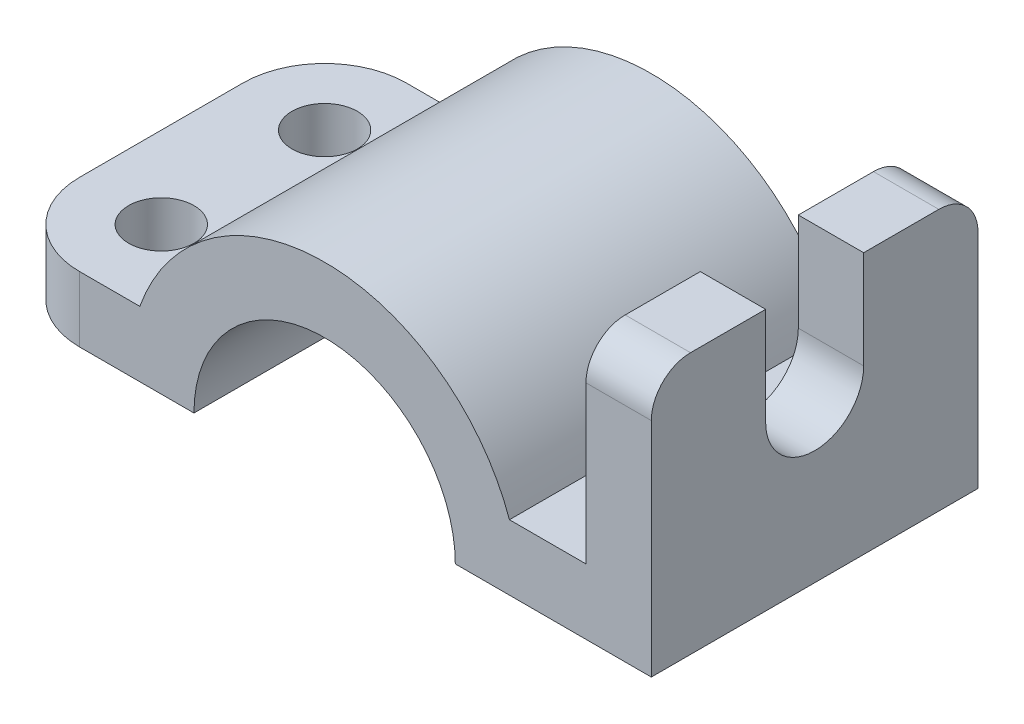
ISO-10303-21;
HEADER;
FILE_DESCRIPTION(('STEP AP214'),'2;1');
FILE_NAME('part.step','',(''),(''),'','','');
FILE_SCHEMA(('AUTOMOTIVE_DESIGN { 1 0 10303 214 1 1 1 1 }'));
ENDSEC;
DATA;
#1=APPLICATION_CONTEXT('core data for automotive mechanical design processes');
#2=APPLICATION_PROTOCOL_DEFINITION('international standard','automotive_design',2000,#1);
#3=PRODUCT_CONTEXT('',#1,'mechanical');
#4=PRODUCT('Part','Part','',(#3));
#5=PRODUCT_RELATED_PRODUCT_CATEGORY('part','',(#4));
#6=PRODUCT_DEFINITION_FORMATION('','',#4);
#7=PRODUCT_DEFINITION_CONTEXT('part definition',#1,'design');
#8=PRODUCT_DEFINITION('design','',#6,#7);
#9=PRODUCT_DEFINITION_SHAPE('','',#8);
#10=(LENGTH_UNIT() NAMED_UNIT(*) SI_UNIT(.MILLI.,.METRE.));
#11=(NAMED_UNIT(*) PLANE_ANGLE_UNIT() SI_UNIT($,.RADIAN.));
#12=(NAMED_UNIT(*) SI_UNIT($,.STERADIAN.) SOLID_ANGLE_UNIT());
#13=UNCERTAINTY_MEASURE_WITH_UNIT(LENGTH_MEASURE(1.E-05),#10,'distance_accuracy_value','');
#14=(GEOMETRIC_REPRESENTATION_CONTEXT(3) GLOBAL_UNCERTAINTY_ASSIGNED_CONTEXT((#13)) GLOBAL_UNIT_ASSIGNED_CONTEXT((#10,
#11,#12)) REPRESENTATION_CONTEXT('',''));
#15=CARTESIAN_POINT('',(0.,0.,0.));
#16=DIRECTION('',(0.,0.,1.));
#17=DIRECTION('',(1.,0.,0.));
#18=AXIS2_PLACEMENT_3D('',#15,#16,#17);
#19=CARTESIAN_POINT('',(50.,40.,25.));
#20=DIRECTION('',(-1.,0.,0.));
#21=DIRECTION('',(0.,-1.,0.));
#22=AXIS2_PLACEMENT_3D('',#19,#20,#21);
#23=PLANE('',#22);
#24=DIRECTION('',(0.,-1.,0.));
#25=VECTOR('',#24,1.);
#26=CARTESIAN_POINT('',(50.,40.,7.5));
#27=LINE('',#26,#25);
#28=CARTESIAN_POINT('',(50.,40.,7.5));
#29=VERTEX_POINT('',#28);
#30=CARTESIAN_POINT('',(50.000006,25.,7.5));
#31=VERTEX_POINT('',#30);
#32=EDGE_CURVE('E374',#29,#31,#27,.T.);
#33=ORIENTED_EDGE('',*,*,#32,.F.);
#34=DIRECTION('',(0.,0.,-1.));
#35=VECTOR('',#34,1.);
#36=CARTESIAN_POINT('',(50.,40.,25.));
#37=LINE('',#36,#35);
#38=CARTESIAN_POINT('',(50.,40.,19.));
#39=VERTEX_POINT('',#38);
#40=EDGE_CURVE('E272',#39,#29,#37,.T.);
#41=ORIENTED_EDGE('',*,*,#40,.F.);
#42=CARTESIAN_POINT('',(50.,34.,19.));
#43=DIRECTION('',(-1.,0.,0.));
#44=DIRECTION('',(0.,-1.,0.));
#45=AXIS2_PLACEMENT_3D('',#42,#43,#44);
#46=CIRCLE('',#45,6.);
#47=CARTESIAN_POINT('',(50.,34.,25.));
#48=VERTEX_POINT('',#47);
#49=EDGE_CURVE('E178',#39,#48,#46,.F.);
#50=ORIENTED_EDGE('',*,*,#49,.T.);
#51=DIRECTION('',(0.,1.,0.));
#52=VECTOR('',#51,1.);
#53=CARTESIAN_POINT('',(50.,40.,25.));
#54=LINE('',#53,#52);
#55=CARTESIAN_POINT('',(50.,0.,25.));
#56=VERTEX_POINT('',#55);
#57=EDGE_CURVE('E271',#56,#48,#54,.T.);
#58=ORIENTED_EDGE('',*,*,#57,.F.);
#59=DIRECTION('',(0.,0.,-1.));
#60=VECTOR('',#59,1.);
#61=CARTESIAN_POINT('',(50.,0.,25.));
#62=LINE('',#61,#60);
#63=CARTESIAN_POINT('',(50.,0.,-25.));
#64=VERTEX_POINT('',#63);
#65=EDGE_CURVE('E190',#56,#64,#62,.T.);
#66=ORIENTED_EDGE('',*,*,#65,.T.);
#67=DIRECTION('',(0.,1.,0.));
#68=VECTOR('',#67,1.);
#69=CARTESIAN_POINT('',(50.,40.,-25.));
#70=LINE('',#69,#68);
#71=CARTESIAN_POINT('',(50.,34.,-25.));
#72=VERTEX_POINT('',#71);
#73=EDGE_CURVE('E168',#64,#72,#70,.T.);
#74=ORIENTED_EDGE('',*,*,#73,.T.);
#75=CARTESIAN_POINT('',(50.,34.,-19.));
#76=DIRECTION('',(-1.,0.,0.));
#77=DIRECTION('',(0.,-1.,0.));
#78=AXIS2_PLACEMENT_3D('',#75,#76,#77);
#79=CIRCLE('',#78,6.);
#80=CARTESIAN_POINT('',(50.,40.,-19.));
#81=VERTEX_POINT('',#80);
#82=EDGE_CURVE('E51',#72,#81,#79,.F.);
#83=ORIENTED_EDGE('',*,*,#82,.T.);
#84=DIRECTION('',(0.,0.,-1.));
#85=VECTOR('',#84,1.);
#86=CARTESIAN_POINT('',(50.,40.,25.));
#87=LINE('',#86,#85);
#88=CARTESIAN_POINT('',(50.,40.,-7.5));
#89=VERTEX_POINT('',#88);
#90=EDGE_CURVE('E44',#89,#81,#87,.T.);
#91=ORIENTED_EDGE('',*,*,#90,.F.);
#92=DIRECTION('',(0.,1.,0.));
#93=VECTOR('',#92,1.);
#94=CARTESIAN_POINT('',(50.,40.,-7.5));
#95=LINE('',#94,#93);
#96=CARTESIAN_POINT('',(50.,25.,-7.5));
#97=VERTEX_POINT('',#96);
#98=EDGE_CURVE('E77',#97,#89,#95,.T.);
#99=ORIENTED_EDGE('',*,*,#98,.F.);
#100=CARTESIAN_POINT('',(50.000012,25.,0.));
#101=DIRECTION('',(1.,0.,0.));
#102=DIRECTION('',(0.,0.,1.));
#103=AXIS2_PLACEMENT_3D('',#100,#101,#102);
#104=CIRCLE('',#103,7.5);
#105=EDGE_CURVE('E205',#31,#97,#104,.T.);
#106=ORIENTED_EDGE('',*,*,#105,.F.);
#107=EDGE_LOOP('',(#33,#41,#50,#58,#66,#74,#83,#91,#99,#106));
#108=FACE_BOUND('',#107,.T.);
#109=ADVANCED_FACE('F41',(#108),#23,.F.);
#110=CARTESIAN_POINT('',(50.,40.,25.));
#111=DIRECTION('',(0.,-1.,0.));
#112=DIRECTION('',(0.,0.,-1.));
#113=AXIS2_PLACEMENT_3D('',#110,#111,#112);
#114=PLANE('',#113);
#115=DIRECTION('',(-1.,0.,0.));
#116=VECTOR('',#115,1.);
#117=CARTESIAN_POINT('',(50.000012,40.,-7.5));
#118=LINE('',#117,#116);
#119=CARTESIAN_POINT('',(40.,40.,-7.5));
#120=VERTEX_POINT('',#119);
#121=EDGE_CURVE('E365',#89,#120,#118,.T.);
#122=ORIENTED_EDGE('',*,*,#121,.F.);
#123=ORIENTED_EDGE('',*,*,#90,.T.);
#124=DIRECTION('',(-1.,0.,0.));
#125=VECTOR('',#124,1.);
#126=CARTESIAN_POINT('',(40.,40.,-19.));
#127=LINE('',#126,#125);
#128=CARTESIAN_POINT('',(40.,40.,-19.));
#129=VERTEX_POINT('',#128);
#130=EDGE_CURVE('E194',#81,#129,#127,.T.);
#131=ORIENTED_EDGE('',*,*,#130,.T.);
#132=DIRECTION('',(0.,0.,-1.));
#133=VECTOR('',#132,1.);
#134=CARTESIAN_POINT('',(40.,40.,25.));
#135=LINE('',#134,#133);
#136=EDGE_CURVE('E309',#120,#129,#135,.T.);
#137=ORIENTED_EDGE('',*,*,#136,.F.);
#138=EDGE_LOOP('',(#122,#123,#131,#137));
#139=FACE_BOUND('',#138,.T.);
#140=ADVANCED_FACE('F220',(#139),#114,.F.);
#141=CARTESIAN_POINT('',(40.,40.,25.));
#142=DIRECTION('',(1.,0.,0.));
#143=DIRECTION('',(0.,1.,0.));
#144=AXIS2_PLACEMENT_3D('',#141,#142,#143);
#145=PLANE('',#144);
#146=DIRECTION('',(0.,-1.,0.));
#147=VECTOR('',#146,1.);
#148=CARTESIAN_POINT('',(40.,40.,-7.5));
#149=LINE('',#148,#147);
#150=CARTESIAN_POINT('',(40.,25.,-7.5));
#151=VERTEX_POINT('',#150);
#152=EDGE_CURVE('E58',#120,#151,#149,.T.);
#153=ORIENTED_EDGE('',*,*,#152,.F.);
#154=ORIENTED_EDGE('',*,*,#136,.T.);
#155=CARTESIAN_POINT('',(40.,34.,-19.));
#156=DIRECTION('',(1.,0.,0.));
#157=DIRECTION('',(0.,1.,0.));
#158=AXIS2_PLACEMENT_3D('',#155,#156,#157);
#159=CIRCLE('',#158,6.);
#160=CARTESIAN_POINT('',(40.,34.,-25.));
#161=VERTEX_POINT('',#160);
#162=EDGE_CURVE('E179',#129,#161,#159,.F.);
#163=ORIENTED_EDGE('',*,*,#162,.T.);
#164=DIRECTION('',(0.,-1.,0.));
#165=VECTOR('',#164,1.);
#166=CARTESIAN_POINT('',(40.,40.,-25.));
#167=LINE('',#166,#165);
#168=CARTESIAN_POINT('',(40.,9.99999999999999,-25.));
#169=VERTEX_POINT('',#168);
#170=EDGE_CURVE('E175',#161,#169,#167,.T.);
#171=ORIENTED_EDGE('',*,*,#170,.T.);
#172=DIRECTION('',(0.,0.,-1.));
#173=VECTOR('',#172,1.);
#174=CARTESIAN_POINT('',(40.,9.99999999999999,25.));
#175=LINE('',#174,#173);
#176=CARTESIAN_POINT('',(40.,9.99999999999999,25.));
#177=VERTEX_POINT('',#176);
#178=EDGE_CURVE('E307',#177,#169,#175,.T.);
#179=ORIENTED_EDGE('',*,*,#178,.F.);
#180=DIRECTION('',(0.,-1.,0.));
#181=VECTOR('',#180,1.);
#182=CARTESIAN_POINT('',(40.,40.,25.));
#183=LINE('',#182,#181);
#184=CARTESIAN_POINT('',(40.,34.,25.));
#185=VERTEX_POINT('',#184);
#186=EDGE_CURVE('E276',#185,#177,#183,.T.);
#187=ORIENTED_EDGE('',*,*,#186,.F.);
#188=CARTESIAN_POINT('',(40.,34.,19.));
#189=DIRECTION('',(1.,0.,0.));
#190=DIRECTION('',(0.,1.,0.));
#191=AXIS2_PLACEMENT_3D('',#188,#189,#190);
#192=CIRCLE('',#191,6.);
#193=CARTESIAN_POINT('',(40.,40.,19.));
#194=VERTEX_POINT('',#193);
#195=EDGE_CURVE('E196',#185,#194,#192,.F.);
#196=ORIENTED_EDGE('',*,*,#195,.T.);
#197=CARTESIAN_POINT('',(40.,40.,7.5));
#198=VERTEX_POINT('',#197);
#199=EDGE_CURVE('E313',#194,#198,#135,.T.);
#200=ORIENTED_EDGE('',*,*,#199,.T.);
#201=DIRECTION('',(0.,1.,0.));
#202=VECTOR('',#201,1.);
#203=CARTESIAN_POINT('',(40.,40.,7.5));
#204=LINE('',#203,#202);
#205=CARTESIAN_POINT('',(40.,25.,7.5));
#206=VERTEX_POINT('',#205);
#207=EDGE_CURVE('E357',#206,#198,#204,.T.);
#208=ORIENTED_EDGE('',*,*,#207,.F.);
#209=CARTESIAN_POINT('',(40.,25.,0.));
#210=DIRECTION('',(1.,0.,0.));
#211=DIRECTION('',(0.,1.,0.));
#212=AXIS2_PLACEMENT_3D('',#209,#210,#211);
#213=CIRCLE('',#212,7.5);
#214=EDGE_CURVE('E367',#151,#206,#213,.F.);
#215=ORIENTED_EDGE('',*,*,#214,.F.);
#216=EDGE_LOOP('',(#153,#154,#163,#171,#179,#187,#196,#200,#208,#215));
#217=FACE_BOUND('',#216,.T.);
#218=ADVANCED_FACE('F241',(#217),#145,.F.);
#219=CARTESIAN_POINT('',(0.,0.,25.));
#220=DIRECTION('',(0.,0.,-1.));
#221=DIRECTION('',(-1.,0.,0.));
#222=AXIS2_PLACEMENT_3D('',#219,#220,#221);
#223=CYLINDRICAL_SURFACE('',#222,30.);
#224=CARTESIAN_POINT('',(0.,0.,-25.));
#225=DIRECTION('',(0.,0.,1.));
#226=DIRECTION('',(-1.,0.,0.));
#227=AXIS2_PLACEMENT_3D('',#224,#225,#226);
#228=CIRCLE('',#227,30.);
#229=CARTESIAN_POINT('',(28.2842712474619,9.99999999999999,-25.));
#230=VERTEX_POINT('',#229);
#231=CARTESIAN_POINT('',(-28.2842712474619,9.99999999999999,-25.));
#232=VERTEX_POINT('',#231);
#233=EDGE_CURVE('E290',#230,#232,#228,.T.);
#234=ORIENTED_EDGE('',*,*,#233,.T.);
#235=DIRECTION('',(0.,0.,-1.));
#236=VECTOR('',#235,1.);
#237=CARTESIAN_POINT('',(-28.2842712474619,9.99999999999999,25.));
#238=LINE('',#237,#236);
#239=CARTESIAN_POINT('',(-28.2842712474619,9.99999999999999,25.));
#240=VERTEX_POINT('',#239);
#241=EDGE_CURVE('E330',#240,#232,#238,.T.);
#242=ORIENTED_EDGE('',*,*,#241,.F.);
#243=CARTESIAN_POINT('',(0.,0.,25.));
#244=DIRECTION('',(0.,0.,1.));
#245=DIRECTION('',(-1.,0.,0.));
#246=AXIS2_PLACEMENT_3D('',#243,#244,#245);
#247=CIRCLE('',#246,30.);
#248=CARTESIAN_POINT('',(28.2842712474619,9.99999999999999,25.));
#249=VERTEX_POINT('',#248);
#250=EDGE_CURVE('E305',#249,#240,#247,.T.);
#251=ORIENTED_EDGE('',*,*,#250,.F.);
#252=DIRECTION('',(0.,0.,-1.));
#253=VECTOR('',#252,1.);
#254=CARTESIAN_POINT('',(28.2842712474619,9.99999999999999,25.));
#255=LINE('',#254,#253);
#256=EDGE_CURVE('E287',#249,#230,#255,.T.);
#257=ORIENTED_EDGE('',*,*,#256,.T.);
#258=EDGE_LOOP('',(#234,#242,#251,#257));
#259=FACE_BOUND('',#258,.T.);
#260=ADVANCED_FACE('F239',(#259),#223,.T.);
#261=CARTESIAN_POINT('',(-50.,10.,25.));
#262=DIRECTION('',(0.,-1.,0.));
#263=DIRECTION('',(1.,0.,0.));
#264=AXIS2_PLACEMENT_3D('',#261,#262,#263);
#265=PLANE('',#264);
#266=CARTESIAN_POINT('',(-37.5,9.99999999999999,12.5));
#267=DIRECTION('',(0.,-1.,0.));
#268=DIRECTION('',(1.,0.,0.));
#269=AXIS2_PLACEMENT_3D('',#266,#267,#268);
#270=CIRCLE('',#269,5.);
#271=CARTESIAN_POINT('',(-32.5,9.99999999999999,12.5));
#272=VERTEX_POINT('',#271);
#273=EDGE_CURVE('E291',#272,#272,#270,.T.);
#274=ORIENTED_EDGE('',*,*,#273,.T.);
#275=EDGE_LOOP('',(#274));
#276=FACE_BOUND('',#275,.T.);
#277=CARTESIAN_POINT('',(-37.5,9.99999999999999,-12.5));
#278=DIRECTION('',(0.,-1.,0.));
#279=DIRECTION('',(1.,0.,0.));
#280=AXIS2_PLACEMENT_3D('',#277,#278,#279);
#281=CIRCLE('',#280,5.);
#282=CARTESIAN_POINT('',(-32.5,9.99999999999999,-12.5));
#283=VERTEX_POINT('',#282);
#284=EDGE_CURVE('E583',#283,#283,#281,.T.);
#285=ORIENTED_EDGE('',*,*,#284,.T.);
#286=EDGE_LOOP('',(#285));
#287=FACE_BOUND('',#286,.T.);
#288=DIRECTION('',(-1.,0.,0.));
#289=VECTOR('',#288,1.);
#290=CARTESIAN_POINT('',(-50.,10.,-25.));
#291=LINE('',#290,#289);
#292=CARTESIAN_POINT('',(-37.5,9.99999999999999,-25.));
#293=VERTEX_POINT('',#292);
#294=EDGE_CURVE('E295',#232,#293,#291,.T.);
#295=ORIENTED_EDGE('',*,*,#294,.T.);
#296=CARTESIAN_POINT('',(-37.5,9.99999999999999,-12.5));
#297=DIRECTION('',(0.,-1.,0.));
#298=DIRECTION('',(1.,0.,0.));
#299=AXIS2_PLACEMENT_3D('',#296,#297,#298);
#300=CIRCLE('',#299,12.5);
#301=CARTESIAN_POINT('',(-50.,10.,-12.5));
#302=VERTEX_POINT('',#301);
#303=EDGE_CURVE('E342',#293,#302,#300,.F.);
#304=ORIENTED_EDGE('',*,*,#303,.T.);
#305=DIRECTION('',(0.,0.,-1.));
#306=VECTOR('',#305,1.);
#307=CARTESIAN_POINT('',(-50.,10.,25.));
#308=LINE('',#307,#306);
#309=CARTESIAN_POINT('',(-50.,10.,12.5));
#310=VERTEX_POINT('',#309);
#311=EDGE_CURVE('E322',#310,#302,#308,.T.);
#312=ORIENTED_EDGE('',*,*,#311,.F.);
#313=CARTESIAN_POINT('',(-37.5,9.99999999999999,12.5));
#314=DIRECTION('',(0.,-1.,0.));
#315=DIRECTION('',(1.,0.,0.));
#316=AXIS2_PLACEMENT_3D('',#313,#314,#315);
#317=CIRCLE('',#316,12.5);
#318=CARTESIAN_POINT('',(-37.5,9.99999999999999,25.));
#319=VERTEX_POINT('',#318);
#320=EDGE_CURVE('E343',#310,#319,#317,.F.);
#321=ORIENTED_EDGE('',*,*,#320,.T.);
#322=DIRECTION('',(-1.,0.,0.));
#323=VECTOR('',#322,1.);
#324=CARTESIAN_POINT('',(-50.,10.,25.));
#325=LINE('',#324,#323);
#326=EDGE_CURVE('E563',#240,#319,#325,.T.);
#327=ORIENTED_EDGE('',*,*,#326,.F.);
#328=ORIENTED_EDGE('',*,*,#241,.T.);
#329=EDGE_LOOP('',(#295,#304,#312,#321,#327,#328));
#330=FACE_BOUND('',#329,.T.);
#331=ADVANCED_FACE('F231',(#276,#287,#330),#265,.F.);
#332=CARTESIAN_POINT('',(-50.,0.,25.));
#333=DIRECTION('',(1.,0.,0.));
#334=DIRECTION('',(0.,0.,-1.));
#335=AXIS2_PLACEMENT_3D('',#332,#333,#334);
#336=PLANE('',#335);
#337=ORIENTED_EDGE('',*,*,#311,.T.);
#338=DIRECTION('',(0.,-1.,0.));
#339=VECTOR('',#338,1.);
#340=CARTESIAN_POINT('',(-50.,0.,-12.5));
#341=LINE('',#340,#339);
#342=CARTESIAN_POINT('',(-50.,0.,-12.5));
#343=VERTEX_POINT('',#342);
#344=EDGE_CURVE('E335',#302,#343,#341,.T.);
#345=ORIENTED_EDGE('',*,*,#344,.T.);
#346=DIRECTION('',(0.,0.,-1.));
#347=VECTOR('',#346,1.);
#348=CARTESIAN_POINT('',(-50.,0.,25.));
#349=LINE('',#348,#347);
#350=CARTESIAN_POINT('',(-50.,0.,12.5));
#351=VERTEX_POINT('',#350);
#352=EDGE_CURVE('E321',#351,#343,#349,.T.);
#353=ORIENTED_EDGE('',*,*,#352,.F.);
#354=DIRECTION('',(0.,-1.,0.));
#355=VECTOR('',#354,1.);
#356=CARTESIAN_POINT('',(-50.,0.,12.5));
#357=LINE('',#356,#355);
#358=EDGE_CURVE('E329',#351,#310,#357,.F.);
#359=ORIENTED_EDGE('',*,*,#358,.T.);
#360=EDGE_LOOP('',(#337,#345,#353,#359));
#361=FACE_BOUND('',#360,.T.);
#362=ADVANCED_FACE('F233',(#361),#336,.F.);
#363=CARTESIAN_POINT('',(-20.,0.,25.));
#364=DIRECTION('',(0.,1.,0.));
#365=DIRECTION('',(-1.,0.,0.));
#366=AXIS2_PLACEMENT_3D('',#363,#364,#365);
#367=PLANE('',#366);
#368=CARTESIAN_POINT('',(-37.5,0.,12.5));
#369=DIRECTION('',(0.,1.,0.));
#370=DIRECTION('',(-1.,0.,0.));
#371=AXIS2_PLACEMENT_3D('',#368,#369,#370);
#372=CIRCLE('',#371,5.);
#373=CARTESIAN_POINT('',(-42.5,0.,12.5));
#374=VERTEX_POINT('',#373);
#375=EDGE_CURVE('E392',#374,#374,#372,.T.);
#376=ORIENTED_EDGE('',*,*,#375,.T.);
#377=EDGE_LOOP('',(#376));
#378=FACE_BOUND('',#377,.T.);
#379=CARTESIAN_POINT('',(-37.5,0.,-12.5));
#380=DIRECTION('',(0.,1.,0.));
#381=DIRECTION('',(-1.,0.,0.));
#382=AXIS2_PLACEMENT_3D('',#379,#380,#381);
#383=CIRCLE('',#382,5.);
#384=CARTESIAN_POINT('',(-42.5,0.,-12.5));
#385=VERTEX_POINT('',#384);
#386=EDGE_CURVE('E389',#385,#385,#383,.T.);
#387=ORIENTED_EDGE('',*,*,#386,.T.);
#388=EDGE_LOOP('',(#387));
#389=FACE_BOUND('',#388,.T.);
#390=ORIENTED_EDGE('',*,*,#352,.T.);
#391=CARTESIAN_POINT('',(-37.5,0.,-12.5));
#392=DIRECTION('',(0.,1.,0.));
#393=DIRECTION('',(-1.,0.,0.));
#394=AXIS2_PLACEMENT_3D('',#391,#392,#393);
#395=CIRCLE('',#394,12.5);
#396=CARTESIAN_POINT('',(-37.5,0.,-25.));
#397=VERTEX_POINT('',#396);
#398=EDGE_CURVE('E340',#343,#397,#395,.F.);
#399=ORIENTED_EDGE('',*,*,#398,.T.);
#400=DIRECTION('',(1.,0.,0.));
#401=VECTOR('',#400,1.);
#402=CARTESIAN_POINT('',(-20.,0.,-25.));
#403=LINE('',#402,#401);
#404=CARTESIAN_POINT('',(-20.,0.,-25.));
#405=VERTEX_POINT('',#404);
#406=EDGE_CURVE('E298',#397,#405,#403,.T.);
#407=ORIENTED_EDGE('',*,*,#406,.T.);
#408=DIRECTION('',(0.,0.,-1.));
#409=VECTOR('',#408,1.);
#410=CARTESIAN_POINT('',(-20.,0.,25.));
#411=LINE('',#410,#409);
#412=CARTESIAN_POINT('',(-20.,0.,25.));
#413=VERTEX_POINT('',#412);
#414=EDGE_CURVE('E318',#413,#405,#411,.T.);
#415=ORIENTED_EDGE('',*,*,#414,.F.);
#416=DIRECTION('',(1.,0.,0.));
#417=VECTOR('',#416,1.);
#418=CARTESIAN_POINT('',(-20.,0.,25.));
#419=LINE('',#418,#417);
#420=CARTESIAN_POINT('',(-37.5,0.,25.));
#421=VERTEX_POINT('',#420);
#422=EDGE_CURVE('E561',#421,#413,#419,.T.);
#423=ORIENTED_EDGE('',*,*,#422,.F.);
#424=CARTESIAN_POINT('',(-37.5,0.,12.5));
#425=DIRECTION('',(0.,1.,0.));
#426=DIRECTION('',(-1.,0.,0.));
#427=AXIS2_PLACEMENT_3D('',#424,#425,#426);
#428=CIRCLE('',#427,12.5);
#429=EDGE_CURVE('E333',#421,#351,#428,.F.);
#430=ORIENTED_EDGE('',*,*,#429,.T.);
#431=EDGE_LOOP('',(#390,#399,#407,#415,#423,#430));
#432=FACE_BOUND('',#431,.T.);
#433=ADVANCED_FACE('F230',(#378,#389,#432),#367,.F.);
#434=CARTESIAN_POINT('',(0.,0.,25.));
#435=DIRECTION('',(0.,0.,-1.));
#436=DIRECTION('',(-1.,0.,0.));
#437=AXIS2_PLACEMENT_3D('',#434,#435,#436);
#438=CYLINDRICAL_SURFACE('',#437,20.);
#439=CARTESIAN_POINT('',(0.,0.,-25.));
#440=DIRECTION('',(0.,0.,-1.));
#441=DIRECTION('',(-1.,0.,0.));
#442=AXIS2_PLACEMENT_3D('',#439,#440,#441);
#443=CIRCLE('',#442,20.);
#444=CARTESIAN_POINT('',(20.,0.,-25.));
#445=VERTEX_POINT('',#444);
#446=EDGE_CURVE('E296',#405,#445,#443,.T.);
#447=ORIENTED_EDGE('',*,*,#446,.T.);
#448=DIRECTION('',(0.,0.,-1.));
#449=VECTOR('',#448,1.);
#450=CARTESIAN_POINT('',(20.,0.,25.));
#451=LINE('',#450,#449);
#452=CARTESIAN_POINT('',(20.,0.,25.));
#453=VERTEX_POINT('',#452);
#454=EDGE_CURVE('E312',#453,#445,#451,.T.);
#455=ORIENTED_EDGE('',*,*,#454,.F.);
#456=CARTESIAN_POINT('',(0.,0.,25.));
#457=DIRECTION('',(0.,0.,-1.));
#458=DIRECTION('',(-1.,0.,0.));
#459=AXIS2_PLACEMENT_3D('',#456,#457,#458);
#460=CIRCLE('',#459,20.);
#461=EDGE_CURVE('E281',#413,#453,#460,.T.);
#462=ORIENTED_EDGE('',*,*,#461,.F.);
#463=ORIENTED_EDGE('',*,*,#414,.T.);
#464=EDGE_LOOP('',(#447,#455,#462,#463));
#465=FACE_BOUND('',#464,.T.);
#466=ADVANCED_FACE('F224',(#465),#438,.F.);
#467=CARTESIAN_POINT('',(50.,0.,25.));
#468=DIRECTION('',(0.,1.,0.));
#469=DIRECTION('',(-1.,0.,0.));
#470=AXIS2_PLACEMENT_3D('',#467,#468,#469);
#471=PLANE('',#470);
#472=DIRECTION('',(1.,0.,0.));
#473=VECTOR('',#472,1.);
#474=CARTESIAN_POINT('',(50.,0.,-25.));
#475=LINE('',#474,#473);
#476=EDGE_CURVE('E186',#445,#64,#475,.T.);
#477=ORIENTED_EDGE('',*,*,#476,.T.);
#478=ORIENTED_EDGE('',*,*,#65,.F.);
#479=DIRECTION('',(1.,0.,0.));
#480=VECTOR('',#479,1.);
#481=CARTESIAN_POINT('',(50.,0.,25.));
#482=LINE('',#481,#480);
#483=EDGE_CURVE('E279',#453,#56,#482,.T.);
#484=ORIENTED_EDGE('',*,*,#483,.F.);
#485=ORIENTED_EDGE('',*,*,#454,.T.);
#486=EDGE_LOOP('',(#477,#478,#484,#485));
#487=FACE_BOUND('',#486,.T.);
#488=ADVANCED_FACE('F219',(#487),#471,.F.);
#489=ORIENTED_EDGE('',*,*,#40,.T.);
#490=DIRECTION('',(-1.,0.,0.));
#491=VECTOR('',#490,1.);
#492=CARTESIAN_POINT('',(50.000012,40.,7.5));
#493=LINE('',#492,#491);
#494=EDGE_CURVE('E355',#29,#198,#493,.T.);
#495=ORIENTED_EDGE('',*,*,#494,.T.);
#496=ORIENTED_EDGE('',*,*,#199,.F.);
#497=DIRECTION('',(-1.,0.,0.));
#498=VECTOR('',#497,1.);
#499=CARTESIAN_POINT('',(50.,40.,19.));
#500=LINE('',#499,#498);
#501=EDGE_CURVE('E200',#194,#39,#500,.F.);
#502=ORIENTED_EDGE('',*,*,#501,.T.);
#503=EDGE_LOOP('',(#489,#495,#496,#502));
#504=FACE_BOUND('',#503,.T.);
#505=ADVANCED_FACE('F217',(#504),#114,.F.);
#506=CARTESIAN_POINT('',(40.,9.99999999999999,25.));
#507=DIRECTION('',(0.,-1.,0.));
#508=DIRECTION('',(1.,0.,0.));
#509=AXIS2_PLACEMENT_3D('',#506,#507,#508);
#510=PLANE('',#509);
#511=DIRECTION('',(-1.,0.,0.));
#512=VECTOR('',#511,1.);
#513=CARTESIAN_POINT('',(40.,9.99999999999999,-25.));
#514=LINE('',#513,#512);
#515=EDGE_CURVE('E304',#169,#230,#514,.T.);
#516=ORIENTED_EDGE('',*,*,#515,.T.);
#517=ORIENTED_EDGE('',*,*,#256,.F.);
#518=DIRECTION('',(-1.,0.,0.));
#519=VECTOR('',#518,1.);
#520=CARTESIAN_POINT('',(40.,9.99999999999999,25.));
#521=LINE('',#520,#519);
#522=EDGE_CURVE('E283',#177,#249,#521,.T.);
#523=ORIENTED_EDGE('',*,*,#522,.F.);
#524=ORIENTED_EDGE('',*,*,#178,.T.);
#525=EDGE_LOOP('',(#516,#517,#523,#524));
#526=FACE_BOUND('',#525,.T.);
#527=ADVANCED_FACE('F415',(#526),#510,.F.);
#528=CARTESIAN_POINT('',(0.,0.,25.));
#529=DIRECTION('',(0.,0.,-1.));
#530=DIRECTION('',(-1.,0.,0.));
#531=AXIS2_PLACEMENT_3D('',#528,#529,#530);
#532=PLANE('',#531);
#533=ORIENTED_EDGE('',*,*,#57,.T.);
#534=DIRECTION('',(-1.,0.,0.));
#535=VECTOR('',#534,1.);
#536=CARTESIAN_POINT('',(0.,34.,25.));
#537=LINE('',#536,#535);
#538=EDGE_CURVE('E11',#48,#185,#537,.T.);
#539=ORIENTED_EDGE('',*,*,#538,.T.);
#540=ORIENTED_EDGE('',*,*,#186,.T.);
#541=ORIENTED_EDGE('',*,*,#522,.T.);
#542=ORIENTED_EDGE('',*,*,#250,.T.);
#543=ORIENTED_EDGE('',*,*,#326,.T.);
#544=DIRECTION('',(0.,-1.,0.));
#545=VECTOR('',#544,1.);
#546=CARTESIAN_POINT('',(-37.5,0.,25.));
#547=LINE('',#546,#545);
#548=EDGE_CURVE('E341',#319,#421,#547,.T.);
#549=ORIENTED_EDGE('',*,*,#548,.T.);
#550=ORIENTED_EDGE('',*,*,#422,.T.);
#551=ORIENTED_EDGE('',*,*,#461,.T.);
#552=ORIENTED_EDGE('',*,*,#483,.T.);
#553=EDGE_LOOP('',(#533,#539,#540,#541,#542,#543,#549,#550,#551,#552));
#554=FACE_BOUND('',#553,.T.);
#555=ADVANCED_FACE('F274',(#554),#532,.F.);
#556=CARTESIAN_POINT('',(0.,0.,-25.));
#557=DIRECTION('',(0.,0.,-1.));
#558=DIRECTION('',(-1.,0.,0.));
#559=AXIS2_PLACEMENT_3D('',#556,#557,#558);
#560=PLANE('',#559);
#561=ORIENTED_EDGE('',*,*,#170,.F.);
#562=DIRECTION('',(-1.,0.,0.));
#563=VECTOR('',#562,1.);
#564=CARTESIAN_POINT('',(50.,34.,-25.));
#565=LINE('',#564,#563);
#566=EDGE_CURVE('E167',#161,#72,#565,.F.);
#567=ORIENTED_EDGE('',*,*,#566,.T.);
#568=ORIENTED_EDGE('',*,*,#73,.F.);
#569=ORIENTED_EDGE('',*,*,#476,.F.);
#570=ORIENTED_EDGE('',*,*,#446,.F.);
#571=ORIENTED_EDGE('',*,*,#406,.F.);
#572=DIRECTION('',(0.,-1.,0.));
#573=VECTOR('',#572,1.);
#574=CARTESIAN_POINT('',(-37.5,10.,-25.));
#575=LINE('',#574,#573);
#576=EDGE_CURVE('E337',#397,#293,#575,.F.);
#577=ORIENTED_EDGE('',*,*,#576,.T.);
#578=ORIENTED_EDGE('',*,*,#294,.F.);
#579=ORIENTED_EDGE('',*,*,#233,.F.);
#580=ORIENTED_EDGE('',*,*,#515,.F.);
#581=EDGE_LOOP('',(#561,#567,#568,#569,#570,#571,#577,#578,#579,#580));
#582=FACE_BOUND('',#581,.T.);
#583=ADVANCED_FACE('F169',(#582),#560,.T.);
#584=CARTESIAN_POINT('',(-37.5,0.,-12.5));
#585=DIRECTION('',(0.,1.,0.));
#586=DIRECTION('',(0.,0.,1.));
#587=AXIS2_PLACEMENT_3D('',#584,#585,#586);
#588=CYLINDRICAL_SURFACE('',#587,12.5);
#589=ORIENTED_EDGE('',*,*,#303,.F.);
#590=ORIENTED_EDGE('',*,*,#576,.F.);
#591=ORIENTED_EDGE('',*,*,#398,.F.);
#592=ORIENTED_EDGE('',*,*,#344,.F.);
#593=EDGE_LOOP('',(#589,#590,#591,#592));
#594=FACE_BOUND('',#593,.T.);
#595=ADVANCED_FACE('F244',(#594),#588,.T.);
#596=CARTESIAN_POINT('',(-37.5,0.,12.5));
#597=DIRECTION('',(0.,-1.,0.));
#598=DIRECTION('',(0.,0.,-1.));
#599=AXIS2_PLACEMENT_3D('',#596,#597,#598);
#600=CYLINDRICAL_SURFACE('',#599,12.5);
#601=ORIENTED_EDGE('',*,*,#320,.F.);
#602=ORIENTED_EDGE('',*,*,#358,.F.);
#603=ORIENTED_EDGE('',*,*,#429,.F.);
#604=ORIENTED_EDGE('',*,*,#548,.F.);
#605=EDGE_LOOP('',(#601,#602,#603,#604));
#606=FACE_BOUND('',#605,.T.);
#607=ADVANCED_FACE('F247',(#606),#600,.T.);
#608=CARTESIAN_POINT('',(50.,34.,-19.));
#609=DIRECTION('',(1.,0.,0.));
#610=DIRECTION('',(0.,0.,-1.));
#611=AXIS2_PLACEMENT_3D('',#608,#609,#610);
#612=CYLINDRICAL_SURFACE('',#611,6.);
#613=ORIENTED_EDGE('',*,*,#82,.F.);
#614=ORIENTED_EDGE('',*,*,#566,.F.);
#615=ORIENTED_EDGE('',*,*,#162,.F.);
#616=ORIENTED_EDGE('',*,*,#130,.F.);
#617=EDGE_LOOP('',(#613,#614,#615,#616));
#618=FACE_BOUND('',#617,.T.);
#619=ADVANCED_FACE('F189',(#618),#612,.T.);
#620=CARTESIAN_POINT('',(0.,34.,19.));
#621=DIRECTION('',(-1.,0.,0.));
#622=DIRECTION('',(0.,0.,1.));
#623=AXIS2_PLACEMENT_3D('',#620,#621,#622);
#624=CYLINDRICAL_SURFACE('',#623,6.);
#625=ORIENTED_EDGE('',*,*,#49,.F.);
#626=ORIENTED_EDGE('',*,*,#501,.F.);
#627=ORIENTED_EDGE('',*,*,#195,.F.);
#628=ORIENTED_EDGE('',*,*,#538,.F.);
#629=EDGE_LOOP('',(#625,#626,#627,#628));
#630=FACE_BOUND('',#629,.T.);
#631=ADVANCED_FACE('F43',(#630),#624,.T.);
#632=CARTESIAN_POINT('',(-37.5,0.,-12.5));
#633=DIRECTION('',(0.,1.,0.));
#634=DIRECTION('',(-1.,0.,0.));
#635=AXIS2_PLACEMENT_3D('',#632,#633,#634);
#636=CYLINDRICAL_SURFACE('',#635,5.);
#637=ORIENTED_EDGE('',*,*,#386,.F.);
#638=EDGE_LOOP('',(#637));
#639=FACE_BOUND('',#638,.T.);
#640=ORIENTED_EDGE('',*,*,#284,.F.);
#641=EDGE_LOOP('',(#640));
#642=FACE_BOUND('',#641,.T.);
#643=ADVANCED_FACE('F260',(#639,#642),#636,.F.);
#644=CARTESIAN_POINT('',(-37.5,0.,12.5));
#645=DIRECTION('',(0.,1.,0.));
#646=DIRECTION('',(-1.,0.,0.));
#647=AXIS2_PLACEMENT_3D('',#644,#645,#646);
#648=CYLINDRICAL_SURFACE('',#647,5.);
#649=ORIENTED_EDGE('',*,*,#375,.F.);
#650=EDGE_LOOP('',(#649));
#651=FACE_BOUND('',#650,.T.);
#652=ORIENTED_EDGE('',*,*,#273,.F.);
#653=EDGE_LOOP('',(#652));
#654=FACE_BOUND('',#653,.T.);
#655=ADVANCED_FACE('F263',(#651,#654),#648,.F.);
#656=CARTESIAN_POINT('',(50.000012,40.,7.5));
#657=DIRECTION('',(0.,0.,-1.));
#658=DIRECTION('',(0.,1.,0.));
#659=AXIS2_PLACEMENT_3D('',#656,#657,#658);
#660=PLANE('',#659);
#661=ORIENTED_EDGE('',*,*,#494,.F.);
#662=ORIENTED_EDGE('',*,*,#32,.T.);
#663=DIRECTION('',(1.,0.,0.));
#664=VECTOR('',#663,1.);
#665=CARTESIAN_POINT('',(-50.001,25.,7.5));
#666=LINE('',#665,#664);
#667=EDGE_CURVE('E89',#206,#31,#666,.T.);
#668=ORIENTED_EDGE('',*,*,#667,.F.);
#669=ORIENTED_EDGE('',*,*,#207,.T.);
#670=EDGE_LOOP('',(#661,#662,#668,#669));
#671=FACE_BOUND('',#670,.T.);
#672=ADVANCED_FACE('F410',(#671),#660,.T.);
#673=CARTESIAN_POINT('',(50.000012,40.,-7.5));
#674=DIRECTION('',(0.,0.,1.));
#675=DIRECTION('',(0.,-1.,0.));
#676=AXIS2_PLACEMENT_3D('',#673,#674,#675);
#677=PLANE('',#676);
#678=ORIENTED_EDGE('',*,*,#98,.T.);
#679=ORIENTED_EDGE('',*,*,#121,.T.);
#680=ORIENTED_EDGE('',*,*,#152,.T.);
#681=DIRECTION('',(1.,0.,0.));
#682=VECTOR('',#681,1.);
#683=CARTESIAN_POINT('',(-50.001,25.,-7.5));
#684=LINE('',#683,#682);
#685=EDGE_CURVE('E385',#151,#97,#684,.T.);
#686=ORIENTED_EDGE('',*,*,#685,.T.);
#687=EDGE_LOOP('',(#678,#679,#680,#686));
#688=FACE_BOUND('',#687,.T.);
#689=ADVANCED_FACE('F364',(#688),#677,.T.);
#690=CARTESIAN_POINT('',(-50.001,25.,0.));
#691=DIRECTION('',(1.,0.,0.));
#692=DIRECTION('',(0.,1.,0.));
#693=AXIS2_PLACEMENT_3D('',#690,#691,#692);
#694=CYLINDRICAL_SURFACE('',#693,7.5);
#695=ORIENTED_EDGE('',*,*,#214,.T.);
#696=ORIENTED_EDGE('',*,*,#667,.T.);
#697=ORIENTED_EDGE('',*,*,#105,.T.);
#698=ORIENTED_EDGE('',*,*,#685,.F.);
#699=EDGE_LOOP('',(#695,#696,#697,#698));
#700=FACE_BOUND('',#699,.T.);
#701=ADVANCED_FACE('F398',(#700),#694,.F.);
#702=CLOSED_SHELL('',(#109,#140,#218,#260,#331,#362,#433,#466,#488,#505,#527,#555,#583,#595,
#607,#619,#631,#643,#655,#672,#689,#701));
#703=MANIFOLD_SOLID_BREP('B2',#702);
#704=ADVANCED_BREP_SHAPE_REPRESENTATION('',(#18,#703),#14);
#705=SHAPE_DEFINITION_REPRESENTATION(#9,#704);
ENDSEC;
END-ISO-10303-21;
